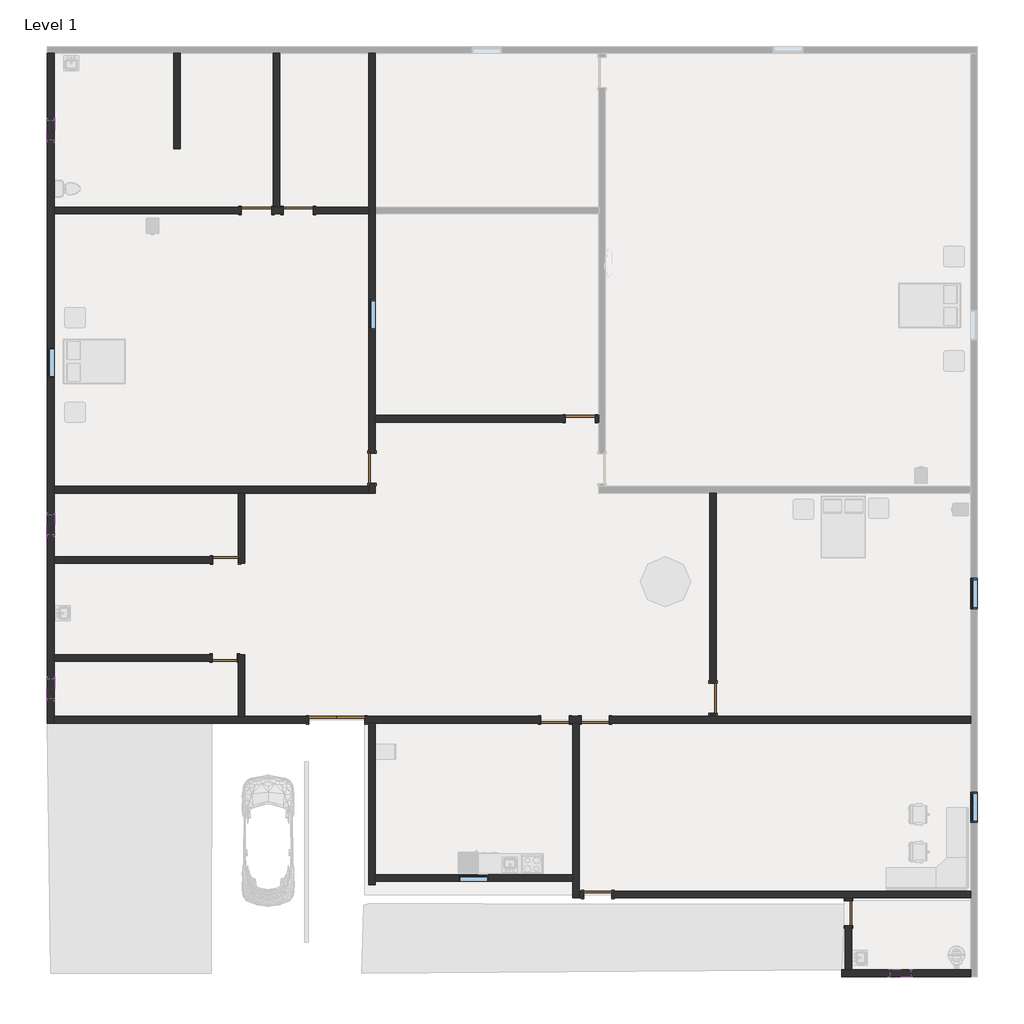
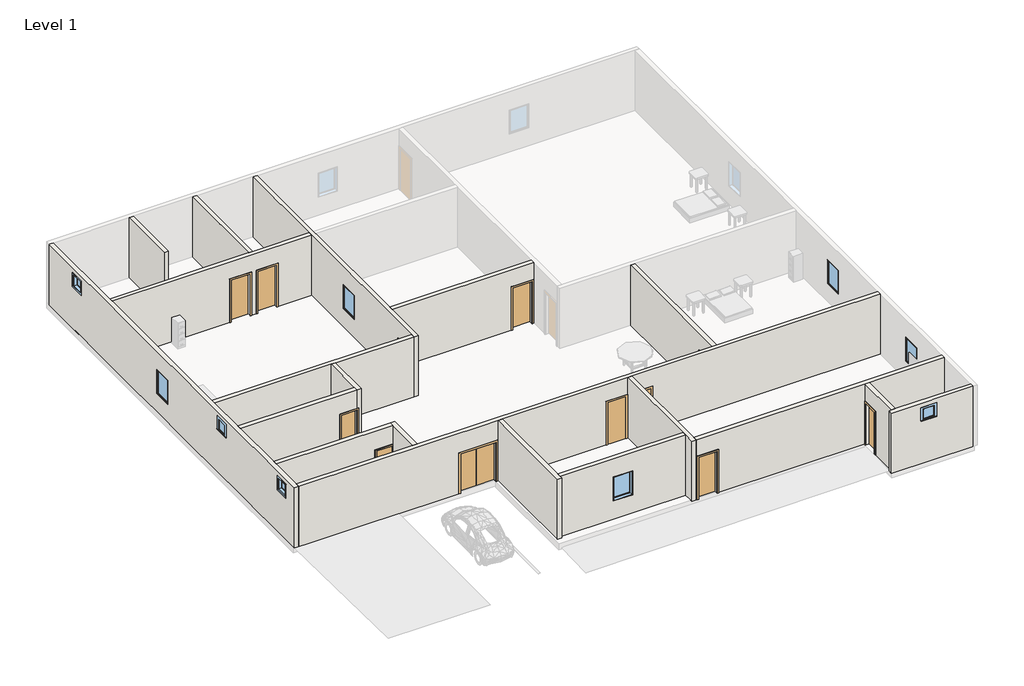
# One storey, part 1 of 2: 19 walls, 12 doors, 9 windows.
"""IFC4 building model written with IfcOpenShell, lengths in millimetres."""

from ifc_helpers import new_model, si_unit, frame, origin, origin_with_axes, place, context, project, spatial, polyline, outline, extrude, faceted_brep, transform, mapped, element, save
from components import m_door_double_flush_panel_1700_x_2000mm_97be971e, door_fadea3f2, door_53b1b562, door_4314e8ec, door_74220ae7, door_f75d31f8, door_54dd4da4, door_719f80de, window_e2841890, window_e41d21a6

model = new_model("IFC4")

# Units and contexts
model_context = context("Model", 3, world=origin())
ifc_project = project(units=[si_unit("LENGTHUNIT", "METRE", prefix="MILLI")], contexts=[model_context])

# Site, building, storey
site = spatial("IfcSite", under=ifc_project)
building = spatial("IfcBuilding", under=site)
storey = spatial("IfcBuildingStorey", under=building, Name="Level 1", Elevation=0.0)

# Doors
placement = place(None, origin())
m_door_double_flush_panel_1700_x_2000mm_shape = m_door_double_flush_panel_1700_x_2000mm_97be971e(model_context)
element("IfcDoor", 1, ObjectType="M_Door-Double-Flush_Panel : 1700 x 2000mm", at=placement, inside=storey, context=model_context, shape_type="MappedRepresentation", body=[
    mapped(m_door_double_flush_panel_1700_x_2000mm_shape, transform((-7405.8725091, -4969.7754008, 0.0), x_axis=(1.0, 0.0, 0.0), y_axis=(0.0, 1.0, 0.0), z_axis=(0.0, 0.0, 1.0))),
])
door_shape = door_fadea3f2(model_context)
element("IfcDoor", 2, ObjectType="Single-Flush : 30\" x 80\"", at=placement, inside=storey, context=model_context, shape_type="MappedRepresentation", body=[
    mapped(door_shape, transform((-10784.0725091, -118.3754008, 0.0), x_axis=(1.0, 0.0, 0.0), y_axis=(0.0, 1.0, 0.0), z_axis=(0.0, 0.0, 1.0))),
])
door_2_shape = door_53b1b562(model_context)
element("IfcDoor", 3, ObjectType="Single-Flush : 30\" x 80\"", at=placement, inside=storey, context=model_context, shape_type="MappedRepresentation", body=[
    mapped(door_2_shape, transform((-10809.4725091, -3090.1754008, 0.0), x_axis=(1.0, 0.0, 0.0), y_axis=(0.0, 1.0, 0.0), z_axis=(0.0, 0.0, 1.0))),
])
door_3_shape = door_4314e8ec(model_context)
element("IfcDoor", 4, ObjectType="Single-Flush : 30\" x 84\"", at=placement, inside=storey, context=model_context, shape_type="MappedRepresentation", body=[
    mapped(door_3_shape, transform((8138.9274909, -10837.1754008, 0.0), x_axis=(0.0, 1.0, 0.0), y_axis=(-1.0, 0.0, 0.0), z_axis=(0.0, 0.0, 1.0))),
])
door_4_shape = door_74220ae7(model_context)
element("IfcDoor", 5, ObjectType="Single-Flush : 34\" x 84\"", at=placement, inside=storey, context=model_context, shape_type="MappedRepresentation", body=[
    mapped(door_4_shape, transform((-776.4725091, -4969.7754008, 0.0), x_axis=(1.0, 0.0, 0.0), y_axis=(0.0, 1.0, 0.0), z_axis=(0.0, 0.0, 1.0))),
])
element("IfcDoor", 6, ObjectType="Single-Flush : 34\" x 84\"", at=placement, inside=storey, context=model_context, shape_type="MappedRepresentation", body=[
    mapped(door_4_shape, transform((518.9274909, -10278.3754008, 0.0), x_axis=(-1.0, 0.0, 0.0), y_axis=(0.0, -1.0, 0.0), z_axis=(0.0, 0.0, 1.0))),
])
door_5_shape = door_f75d31f8(model_context)
element("IfcDoor", 7, ObjectType="Single-Flush : 34\" x 84\"", at=placement, inside=storey, context=model_context, shape_type="MappedRepresentation", body=[
    mapped(door_5_shape, transform((442.7274909, -4969.7754008, 0.0), x_axis=(-1.0, 0.0, 0.0), y_axis=(0.0, -1.0, 0.0), z_axis=(0.0, 0.0, 1.0))),
])
door_6_shape = door_54dd4da4(model_context)
element("IfcDoor", 8, ObjectType="Single-Flush : 36\" x 84\"", at=placement, inside=storey, context=model_context, shape_type="MappedRepresentation", body=[
    mapped(door_6_shape, transform((-9844.2725091, 10498.8245992, 0.0), x_axis=(1.0, 0.0, 0.0), y_axis=(0.0, 1.0, 0.0), z_axis=(0.0, 0.0, 1.0))),
])
element("IfcDoor", 9, ObjectType="Single-Flush : 36\" x 84\"", at=placement, inside=storey, context=model_context, shape_type="MappedRepresentation", body=[
    mapped(door_6_shape, transform((-14.4725091, 4174.2245992, 0.0), x_axis=(1.0, 0.0, 0.0), y_axis=(0.0, 1.0, 0.0), z_axis=(0.0, 0.0, 1.0))),
])
element("IfcDoor", 10, ObjectType="Single-Flush : 36\" x 84\"", at=placement, inside=storey, context=model_context, shape_type="MappedRepresentation", body=[
    mapped(door_6_shape, transform((4024.1274909, -4309.3754008, 0.0), x_axis=(0.0, -1.0, 0.0), y_axis=(1.0, 0.0, 0.0), z_axis=(0.0, 0.0, 1.0))),
])
door_7_shape = door_719f80de(model_context)
element("IfcDoor", 11, ObjectType="Single-Flush : 36\" x 84\"", at=placement, inside=storey, context=model_context, shape_type="MappedRepresentation", body=[
    mapped(door_7_shape, transform((-8574.2725091, 10498.8245992, 0.0), x_axis=(-1.0, 0.0, 0.0), y_axis=(0.0, -1.0, 0.0), z_axis=(0.0, 0.0, 1.0))),
])
element("IfcDoor", 12, ObjectType="Single-Flush : 36\" x 84\"", at=placement, inside=storey, context=model_context, shape_type="MappedRepresentation", body=[
    mapped(door_7_shape, transform((-6339.0725091, 2675.6245992, 0.0), x_axis=(0.0, -1.0, 0.0), y_axis=(1.0, 0.0, 0.0), z_axis=(0.0, 0.0, 1.0))),
])

# Walls
element("IfcWall", 13, ObjectType="Generic - 8\"", at=placement, inside=storey, context=model_context, shape_type="Brep", body=[
    faceted_brep([(11847.3274909, -12564.3754008, 0.0), (8240.5274909, -12564.3754008, 0.0), (8037.3274909, -12564.3754008, 0.0), (7935.7274909, -12564.3754008, 0.0), (7935.7274909, -12564.3754008, 3048.0), (8037.3274909, -12564.3754008, 3048.0), (8240.5274909, -12564.3754008, 3048.0), (11847.3274909, -12564.3754008, 3048.0), (9408.9274909, -12564.3754008, 2768.6), (9408.9274909, -12564.3754008, 2159.0), (10018.5274909, -12564.3754008, 2159.0), (10018.5274909, -12564.3754008, 2768.6), (11847.3274909, -12767.5754008, 0.0), (11847.3274909, -12767.5754008, 3048.0), (7935.7274909, -12767.5754008, 3048.0), (7935.7274909, -12767.5754008, 0.0), (9408.9274909, -12767.5754008, 2768.6), (10018.5274909, -12767.5754008, 2768.6), (10018.5274909, -12767.5754008, 2159.0), (9408.9274909, -12767.5754008, 2159.0)], [[[0, 1, 2, 3, 4, 5, 6, 7], [8, 9, 10, 11]], [[12, 13, 14, 15], [16, 17, 18, 19]], [[3, 2, 1, 0, 12, 15]], [[4, 3, 15, 14]], [[7, 6, 5, 4, 14, 13]], [[0, 7, 13, 12]], [[9, 8, 16, 19]], [[10, 9, 19, 18]], [[11, 10, 18, 17]], [[8, 11, 17, 16]]]),
])
element("IfcWall", 14, ObjectType="Generic - 8\"", at=placement, inside=storey, context=model_context, shape_type="Brep", body=[
    faceted_brep([(-6440.6725091, 2218.4245992, 2133.6), (-6440.6725091, 2218.4245992, 0.0), (-6440.6725091, 2116.8245992, 0.0), (-6440.6725091, 1913.6245992, 0.0), (-6440.6725091, 1913.6245992, 3048.0), (-6440.6725091, 2116.8245992, 3048.0), (-6440.6725091, 10397.2245992, 3048.0), (-6440.6725091, 10600.4245992, 3048.0), (-6440.6725091, 15274.0245992, 3048.0), (-6440.6725091, 15274.0245992, 0.0), (-6440.6725091, 10600.4245992, 0.0), (-6440.6725091, 10397.2245992, 0.0), (-6440.6725091, 3132.8245992, 0.0), (-6440.6725091, 3132.8245992, 2133.6), (-6440.6725091, 7793.7245992, 2133.6), (-6440.6725091, 6879.3245992, 2133.6), (-6440.6725091, 6879.3245992, 914.4), (-6440.6725091, 7793.7245992, 914.4), (-6237.4725091, 1913.6245992, 0.0), (-6237.4725091, 2218.4245992, 0.0), (-6237.4725091, 2218.4245992, 2133.6), (-6237.4725091, 3132.8245992, 2133.6), (-6237.4725091, 3132.8245992, 0.0), (-6237.4725091, 4072.6245992, 0.0), (-6237.4725091, 4275.8245992, 0.0), (-6237.4725091, 10397.2245992, 0.0), (-6237.4725091, 10600.4245992, 0.0), (-6237.4725091, 15274.0245992, 0.0), (-6237.4725091, 15274.0245992, 3048.0), (-6237.4725091, 10600.4245992, 3048.0), (-6237.4725091, 10397.2245992, 3048.0), (-6237.4725091, 4275.8245992, 3048.0), (-6237.4725091, 4072.6245992, 3048.0), (-6237.4725091, 1913.6245992, 3048.0), (-6237.4725091, 7793.7245992, 2133.6), (-6237.4725091, 7793.7245992, 914.4), (-6237.4725091, 6879.3245992, 914.4), (-6237.4725091, 6879.3245992, 2133.6)], [[[0, 1, 2, 3, 4, 5, 6, 7, 8, 9, 10, 11, 12, 13], [14, 15, 16, 17]], [[18, 19, 20, 21, 22, 23, 24, 25, 26, 27, 28, 29, 30, 31, 32, 33], [34, 35, 36, 37]], [[3, 2, 1, 19, 18]], [[12, 11, 10, 9, 27, 26, 25, 24, 23, 22]], [[8, 7, 6, 5, 4, 33, 32, 31, 30, 29, 28]], [[9, 8, 28, 27]], [[4, 3, 18, 33]], [[20, 19, 1, 0]], [[21, 20, 0, 13]], [[22, 21, 13, 12]], [[35, 34, 14, 17]], [[36, 35, 17, 16]], [[37, 36, 16, 15]], [[34, 37, 15, 14]]]),
])
element("IfcWall", 15, ObjectType="Generic - 8\"", at=placement, inside=storey, context=model_context, shape_type="Brep", body=[
    faceted_brep([(-9031.4725091, 10600.4245992, 2133.6), (-9031.4725091, 10600.4245992, 0.0), (-9133.0725091, 10600.4245992, 0.0), (-9336.2725091, 10600.4245992, 0.0), (-9387.0725091, 10600.4245992, 0.0), (-9387.0725091, 10600.4245992, 2133.6), (-10301.4725091, 10600.4245992, 2133.6), (-10301.4725091, 10600.4245992, 0.0), (-15991.0725091, 10600.4245992, 0.0), (-15991.0725091, 10600.4245992, 3048.0), (-9336.2725091, 10600.4245992, 3048.0), (-9133.0725091, 10600.4245992, 3048.0), (-6440.6725091, 10600.4245992, 3048.0), (-6440.6725091, 10600.4245992, 0.0), (-8117.0725091, 10600.4245992, 0.0), (-8117.0725091, 10600.4245992, 2133.6), (-9387.0725091, 10397.2245992, 0.0), (-9031.4725091, 10397.2245992, 0.0), (-9031.4725091, 10397.2245992, 2133.6), (-8117.0725091, 10397.2245992, 2133.6), (-8117.0725091, 10397.2245992, 0.0), (-6440.6725091, 10397.2245992, 0.0), (-6440.6725091, 10397.2245992, 3048.0), (-15991.0725091, 10397.2245992, 3048.0), (-15991.0725091, 10397.2245992, 0.0), (-10301.4725091, 10397.2245992, 0.0), (-10301.4725091, 10397.2245992, 2133.6), (-9387.0725091, 10397.2245992, 2133.6)], [[[0, 1, 2, 3, 4, 5, 6, 7, 8, 9, 10, 11, 12, 13, 14, 15]], [[16, 17, 18, 19, 20, 21, 22, 23, 24, 25, 26, 27]], [[25, 24, 8, 7]], [[14, 13, 21, 20]], [[4, 3, 2, 1, 17, 16]], [[12, 11, 10, 9, 23, 22]], [[13, 12, 22, 21]], [[9, 8, 24, 23]], [[5, 4, 16, 27]], [[6, 5, 27, 26]], [[7, 6, 26, 25]], [[18, 17, 1, 0]], [[19, 18, 0, 15]], [[20, 19, 15, 14]]]),
])
element("IfcWall", 16, ObjectType="Generic - 8\"", at=placement, inside=storey, context=model_context, shape_type="Brep", body=[
    faceted_brep([(-6440.6725091, 2116.8245992, 0.0), (-15991.0725091, 2116.8245992, 0.0), (-15991.0725091, 2116.8245992, 3048.0), (-6440.6725091, 2116.8245992, 3048.0), (-6440.6725091, 1913.6245992, 0.0), (-6440.6725091, 1913.6245992, 3048.0), (-10199.8725091, 1913.6245992, 3048.0), (-10403.0725091, 1913.6245992, 3048.0), (-15991.0725091, 1913.6245992, 3048.0), (-15991.0725091, 1913.6245992, 0.0), (-10403.0725091, 1913.6245992, 0.0), (-10199.8725091, 1913.6245992, 0.0)], [[[0, 1, 2, 3]], [[4, 5, 6, 7, 8, 9, 10, 11]], [[1, 0, 4, 11, 10, 9]], [[3, 2, 8, 7, 6, 5]], [[0, 3, 5, 4]], [[2, 1, 9, 8]]]),
])
element("IfcWall", 17, ObjectType="Generic - 8\"", at=placement, inside=storey, context=model_context, shape_type="Brep", body=[
    faceted_brep([(-10403.0725091, 1913.6245992, 0.0), (-10403.0725091, -219.9754008, 0.0), (-10403.0725091, -219.9754008, 2032.0), (-10403.0725091, -219.9754008, 3048.0), (-10403.0725091, -16.7754008, 3048.0), (-10403.0725091, 1913.6245992, 3048.0), (-10199.8725091, 1913.6245992, 0.0), (-10199.8725091, 1913.6245992, 3048.0), (-10199.8725091, -219.9754008, 3048.0), (-10199.8725091, -219.9754008, 0.0)], [[[0, 1, 2, 3, 4, 5]], [[6, 7, 8, 9]], [[1, 0, 6, 9]], [[5, 4, 3, 8, 7]], [[0, 5, 7, 6]], [[3, 2, 1, 9, 8]]]),
])
element("IfcWall", 18, ObjectType="Generic - 8\"", at=placement, inside=storey, context=model_context, shape_type="Brep", body=[
    faceted_brep([(10.9274909, -4868.1754008, 2133.6), (10.9274909, -4868.1754008, 0.0), (-344.6725091, -4868.1754008, 0.0), (-344.6725091, -4868.1754008, 2133.6), (-1208.2725091, -4868.1754008, 2133.6), (-1208.2725091, -4868.1754008, 0.0), (-6555.8725091, -4868.1754008, 0.0), (-6555.8725091, -4868.1754008, 2000.0), (-8255.8725091, -4868.1754008, 2000.0), (-8255.8725091, -4868.1754008, 0.0), (-10199.8725091, -4868.1754008, 0.0), (-10403.0725091, -4868.1754008, 0.0), (-15991.0725091, -4868.1754008, 0.0), (-15991.0725091, -4868.1754008, 3048.0), (-10403.0725091, -4868.1754008, 3048.0), (-10199.8725091, -4868.1754008, 3048.0), (3922.5274909, -4868.1754008, 3048.0), (4125.7274909, -4868.1754008, 3048.0), (11847.3274909, -4868.1754008, 3048.0), (11847.3274909, -4868.1754008, 0.0), (4125.7274909, -4868.1754008, 0.0), (3922.5274909, -4868.1754008, 0.0), (874.5274909, -4868.1754008, 0.0), (874.5274909, -4868.1754008, 2133.6), (-344.6725091, -5071.3754008, 0.0), (-243.0725091, -5071.3754008, 0.0), (-39.8725091, -5071.3754008, 0.0), (10.9274909, -5071.3754008, 0.0), (10.9274909, -5071.3754008, 2133.6), (874.5274909, -5071.3754008, 2133.6), (874.5274909, -5071.3754008, 0.0), (11847.3274909, -5071.3754008, 0.0), (11847.3274909, -5071.3754008, 3048.0), (-39.8725091, -5071.3754008, 3048.0), (-243.0725091, -5071.3754008, 3048.0), (-6237.4725091, -5071.3754008, 3048.0), (-6440.6725091, -5071.3754008, 3048.0), (-15991.0725091, -5071.3754008, 3048.0), (-15991.0725091, -5071.3754008, 0.0), (-8255.8725091, -5071.3754008, 0.0), (-8255.8725091, -5071.3754008, 2000.0), (-6555.8725091, -5071.3754008, 2000.0), (-6555.8725091, -5071.3754008, 0.0), (-6440.6725091, -5071.3754008, 0.0), (-6237.4725091, -5071.3754008, 0.0), (-1208.2725091, -5071.3754008, 0.0), (-1208.2725091, -5071.3754008, 2133.6), (-344.6725091, -5071.3754008, 2133.6)], [[[0, 1, 2, 3, 4, 5, 6, 7, 8, 9, 10, 11, 12, 13, 14, 15, 16, 17, 18, 19, 20, 21, 22, 23]], [[24, 25, 26, 27, 28, 29, 30, 31, 32, 33, 34, 35, 36, 37, 38, 39, 40, 41, 42, 43, 44, 45, 46, 47]], [[38, 12, 11, 10, 9, 39]], [[45, 44, 43, 42, 6, 5]], [[2, 1, 27, 26, 25, 24]], [[22, 21, 20, 19, 31, 30]], [[18, 17, 16, 15, 14, 13, 37, 36, 35, 34, 33, 32]], [[19, 18, 32, 31]], [[41, 7, 6, 42]], [[7, 41, 40, 8]], [[8, 40, 39, 9]], [[13, 12, 38, 37]], [[3, 2, 24, 47]], [[4, 3, 47, 46]], [[5, 4, 46, 45]], [[28, 27, 1, 0]], [[29, 28, 0, 23]], [[30, 29, 23, 22]]]),
])
element("IfcWall", 19, ObjectType="Generic - 8\"", at=placement, inside=storey, context=model_context, shape_type="Brep", body=[
    faceted_brep([(-6440.6725091, -5071.3754008, 0.0), (-6440.6725091, -9973.5754008, 0.0), (-6440.6725091, -9973.5754008, 3048.0), (-6440.6725091, -5071.3754008, 3048.0), (-6237.4725091, -5071.3754008, 0.0), (-6237.4725091, -5071.3754008, 3048.0), (-6237.4725091, -9668.7754008, 3048.0), (-6237.4725091, -9871.9754008, 3048.0), (-6237.4725091, -9973.5754008, 3048.0), (-6237.4725091, -9973.5754008, 0.0), (-6237.4725091, -9871.9754008, 0.0), (-6237.4725091, -9668.7754008, 0.0)], [[[0, 1, 2, 3]], [[4, 5, 6, 7, 8, 9, 10, 11]], [[1, 0, 4, 11, 10, 9]], [[2, 1, 9, 8]], [[3, 2, 8, 7, 6, 5]], [[0, 3, 5, 4]]]),
])
element("IfcWall", 20, ObjectType="Generic - 8\"", at=placement, inside=storey, context=model_context, shape_type="Brep", body=[
    faceted_brep([(-243.0725091, -5071.3754008, 0.0), (-243.0725091, -9668.7754008, 0.0), (-243.0725091, -9871.9754008, 0.0), (-243.0725091, -10379.9754008, 0.0), (-243.0725091, -10379.9754008, 3048.0), (-243.0725091, -9871.9754008, 3048.0), (-243.0725091, -9668.7754008, 3048.0), (-243.0725091, -5071.3754008, 3048.0), (-39.8725091, -5071.3754008, 0.0), (-39.8725091, -5071.3754008, 3048.0), (-39.8725091, -10176.7754008, 3048.0), (-39.8725091, -10379.9754008, 3048.0), (-39.8725091, -10379.9754008, 0.0), (-39.8725091, -10176.7754008, 0.0)], [[[0, 1, 2, 3, 4, 5, 6, 7]], [[8, 9, 10, 11, 12, 13]], [[3, 2, 1, 0, 8, 13, 12]], [[7, 6, 5, 4, 11, 10, 9]], [[0, 7, 9, 8]], [[4, 3, 12, 11]]]),
])
element("IfcWall", 21, ObjectType="Generic - 8\"", at=placement, inside=storey, context=model_context, shape_type="SweptSolid", body=[
    extrude(outline(polyline([(0.0, -6237.4725091), (0.0, -243.0725091), (3048.0, -243.0725091), (3048.0, -6237.4725091), (0.0, -6237.4725091)]), holes=[polyline([(2133.6, -2783.0725091), (914.4, -2783.0725091), (914.4, -3697.4725091), (2133.6, -3697.4725091), (2133.6, -2783.0725091)])]), frame((0.0, -9871.9754008, 0.0), z_axis=(0.0, 1.0, 0.0), x_axis=(0.0, 0.0, 1.0)), (0.0, 0.0, 1.0), 203.2),
])
element("IfcWall", 22, ObjectType="Generic - 8\"", at=placement, inside=storey, context=model_context, shape_type="Brep", body=[
    faceted_brep([(-39.8725091, -10379.9754008, 0.0), (87.1274909, -10379.9754008, 0.0), (87.1274909, -10379.9754008, 2133.6), (950.7274909, -10379.9754008, 2133.6), (950.7274909, -10379.9754008, 0.0), (8037.3274909, -10379.9754008, 0.0), (8240.5274909, -10379.9754008, 0.0), (11847.3274909, -10379.9754008, 0.0), (11847.3274909, -10379.9754008, 3048.0), (8240.5274909, -10379.9754008, 3048.0), (8037.3274909, -10379.9754008, 3048.0), (-39.8725091, -10379.9754008, 3048.0), (87.1274909, -10176.7754008, 2133.6), (87.1274909, -10176.7754008, 0.0), (-39.8725091, -10176.7754008, 0.0), (-39.8725091, -10176.7754008, 3048.0), (11847.3274909, -10176.7754008, 3048.0), (11847.3274909, -10176.7754008, 0.0), (950.7274909, -10176.7754008, 0.0), (950.7274909, -10176.7754008, 2133.6)], [[[0, 1, 2, 3, 4, 5, 6, 7, 8, 9, 10, 11]], [[12, 13, 14, 15, 16, 17, 18, 19]], [[18, 17, 7, 6, 5, 4]], [[14, 13, 1, 0]], [[11, 10, 9, 8, 16, 15]], [[0, 11, 15, 14]], [[8, 7, 17, 16]], [[2, 1, 13, 12]], [[3, 2, 12, 19]], [[4, 3, 19, 18]]]),
])
element("IfcWall", 23, ObjectType="Generic - 8\"", at=placement, inside=storey, context=model_context, shape_type="SweptSolid", body=[
    extrude(outline(polyline([(-10379.9754008, 0.0), (-10456.1754008, 0.0), (-10456.1754008, 2133.6), (-11218.1754008, 2133.6), (-11218.1754008, 0.0), (-12564.3754008, 0.0), (-12564.3754008, 3048.0), (-10379.9754008, 3048.0), (-10379.9754008, 0.0)])), frame((8037.3274909, 0.0, 0.0), z_axis=(1.0, 0.0, 0.0), x_axis=(0.0, 1.0, 0.0)), (0.0, 0.0, 1.0), 203.2),
])
element("IfcWall", 24, ObjectType="Generic - 8\"", at=placement, inside=storey, context=model_context, shape_type="SweptSolid", body=[
    extrude(outline(polyline([(2133.6, 442.7274909), (0.0, 442.7274909), (0.0, 544.3274909), (3048.0, 544.3274909), (3048.0, -6237.4725091), (0.0, -6237.4725091), (0.0, -471.6725091), (2133.6, -471.6725091), (2133.6, 442.7274909)])), frame((0.0, 4072.6245992, 0.0), z_axis=(0.0, 1.0, 0.0), x_axis=(0.0, 0.0, 1.0)), (0.0, 0.0, 1.0), 203.2),
])
element("IfcWall", 25, ObjectType="Generic - 8\"", at=placement, inside=storey, context=model_context, shape_type="SweptSolid", body=[
    extrude(outline(polyline([(-12358.8725091, 12378.4245992), (-12358.8725091, 15274.0245992), (-12155.6725091, 15274.0245992), (-12155.6725091, 12378.4245992), (-12358.8725091, 12378.4245992)])), origin_with_axes(), (0.0, 0.0, 1.0), 3048.0),
])
element("IfcWall", 26, ObjectType="Generic - 8\"", at=placement, inside=storey, context=model_context, shape_type="SweptSolid", body=[
    extrude(outline(polyline([(-9336.2725091, 10600.4245992), (-9336.2725091, 15274.0245992), (-9133.0725091, 15274.0245992), (-9133.0725091, 10600.4245992), (-9336.2725091, 10600.4245992)])), origin_with_axes(), (0.0, 0.0, 1.0), 3048.0),
])
element("IfcWall", 27, ObjectType="Generic - 8\"", at=placement, inside=storey, context=model_context, shape_type="SweptSolid", body=[
    extrude(outline(polyline([(-4766.5754008, 2133.6), (-4766.5754008, 0.0), (-4868.1754008, 0.0), (-4868.1754008, 3048.0), (1913.6245992, 3048.0), (1913.6245992, 0.0), (-3852.1754008, 0.0), (-3852.1754008, 2133.6), (-4766.5754008, 2133.6)])), frame((3922.5274909, 0.0, 0.0), z_axis=(1.0, 0.0, 0.0), x_axis=(0.0, 1.0, 0.0)), (0.0, 0.0, 1.0), 203.2),
])
element("IfcWall", 28, ObjectType="Generic - 8\"", at=placement, inside=storey, context=model_context, shape_type="Brep", body=[
    faceted_brep([(-10403.0725091, -2988.5754008, 0.0), (-10403.0725091, -3191.7754008, 0.0), (-10403.0725091, -4868.1754008, 0.0), (-10403.0725091, -4868.1754008, 3048.0), (-10403.0725091, -3191.7754008, 3048.0), (-10403.0725091, -2988.5754008, 3048.0), (-10199.8725091, -2988.5754008, 0.0), (-10199.8725091, -2988.5754008, 3048.0), (-10199.8725091, -4868.1754008, 3048.0), (-10199.8725091, -4868.1754008, 0.0)], [[[0, 1, 2, 3, 4, 5]], [[6, 7, 8, 9]], [[2, 1, 0, 6, 9]], [[5, 4, 3, 8, 7]], [[3, 2, 9, 8]], [[0, 5, 7, 6]]]),
])
element("IfcWall", 29, ObjectType="Generic - 8\"", at=placement, inside=storey, context=model_context, shape_type="SweptSolid", body=[
    extrude(outline(polyline([(3048.0, -10403.0725091), (3048.0, -15991.0725091), (0.0, -15991.0725091), (0.0, -11165.0725091), (2032.0, -11165.0725091), (2032.0, -10403.0725091), (3048.0, -10403.0725091)])), frame((0.0, -219.9754008, 0.0), z_axis=(0.0, 1.0, 0.0), x_axis=(0.0, 0.0, 1.0)), (0.0, 0.0, 1.0), 203.2),
])
element("IfcWall", 30, ObjectType="Generic - 8\"", at=placement, inside=storey, context=model_context, shape_type="SweptSolid", body=[
    extrude(outline(polyline([(2032.0, -10428.4725091), (0.0, -10428.4725091), (0.0, -10403.0725091), (3048.0, -10403.0725091), (3048.0, -15991.0725091), (0.0, -15991.0725091), (0.0, -11190.4725091), (2032.0, -11190.4725091), (2032.0, -10428.4725091)])), frame((0.0, -3191.7754008, 0.0), z_axis=(0.0, 1.0, 0.0), x_axis=(0.0, 0.0, 1.0)), (0.0, 0.0, 1.0), 203.2),
])
element("IfcWall", 31, ObjectType="Generic - 8\"", at=placement, inside=storey, context=model_context, shape_type="Brep", body=[
    faceted_brep([(-15991.0725091, -5071.3754008, 0.0), (-15991.0725091, -4868.1754008, 0.0), (-15991.0725091, -3191.7754008, 0.0), (-15991.0725091, -2988.5754008, 0.0), (-15991.0725091, -219.9754008, 0.0), (-15991.0725091, -16.7754008, 0.0), (-15991.0725091, 1913.6245992, 0.0), (-15991.0725091, 2116.8245992, 0.0), (-15991.0725091, 10397.2245992, 0.0), (-15991.0725091, 10600.4245992, 0.0), (-15991.0725091, 15274.0245992, 0.0), (-15991.0725091, 15274.0245992, 3048.0), (-15991.0725091, 10600.4245992, 3048.0), (-15991.0725091, 10397.2245992, 3048.0), (-15991.0725091, 2116.8245992, 3048.0), (-15991.0725091, 1913.6245992, 3048.0), (-15991.0725091, -16.7754008, 3048.0), (-15991.0725091, -219.9754008, 3048.0), (-15991.0725091, -2988.5754008, 3048.0), (-15991.0725091, -3191.7754008, 3048.0), (-15991.0725091, -4868.1754008, 3048.0), (-15991.0725091, -5071.3754008, 3048.0), (-15991.0725091, 6333.2245992, 2133.6), (-15991.0725091, 6333.2245992, 914.4), (-15991.0725091, 5418.8245992, 914.4), (-15991.0725091, 5418.8245992, 2133.6), (-15991.0725091, -4334.7754008, 2768.6), (-15991.0725091, -3725.1754008, 2768.6), (-15991.0725091, -3725.1754008, 2159.0), (-15991.0725091, -4334.7754008, 2159.0), (-15991.0725091, 1253.2245992, 2768.6), (-15991.0725091, 1253.2245992, 2159.0), (-15991.0725091, 643.6245992, 2159.0), (-15991.0725091, 643.6245992, 2768.6), (-15991.0725091, 12632.4245992, 2768.6), (-15991.0725091, 13242.0245992, 2768.6), (-15991.0725091, 13242.0245992, 2159.0), (-15991.0725091, 12632.4245992, 2159.0), (-16194.2725091, -5071.3754008, 0.0), (-16194.2725091, -5071.3754008, 3048.0), (-16194.2725091, 15274.0245992, 3048.0), (-16194.2725091, 15274.0245992, 0.0), (-16194.2725091, 6333.2245992, 2133.6), (-16194.2725091, 5418.8245992, 2133.6), (-16194.2725091, 5418.8245992, 914.4), (-16194.2725091, 6333.2245992, 914.4), (-16194.2725091, -4334.7754008, 2768.6), (-16194.2725091, -4334.7754008, 2159.0), (-16194.2725091, -3725.1754008, 2159.0), (-16194.2725091, -3725.1754008, 2768.6), (-16194.2725091, 1253.2245992, 2768.6), (-16194.2725091, 643.6245992, 2768.6), (-16194.2725091, 643.6245992, 2159.0), (-16194.2725091, 1253.2245992, 2159.0), (-16194.2725091, 12632.4245992, 2768.6), (-16194.2725091, 12632.4245992, 2159.0), (-16194.2725091, 13242.0245992, 2159.0), (-16194.2725091, 13242.0245992, 2768.6)], [[[0, 1, 2, 3, 4, 5, 6, 7, 8, 9, 10, 11, 12, 13, 14, 15, 16, 17, 18, 19, 20, 21], [22, 23, 24, 25], [26, 27, 28, 29], [30, 31, 32, 33], [34, 35, 36, 37]], [[38, 39, 40, 41], [42, 43, 44, 45], [46, 47, 48, 49], [50, 51, 52, 53], [54, 55, 56, 57]], [[10, 9, 8, 7, 6, 5, 4, 3, 2, 1, 0, 38, 41]], [[21, 20, 19, 18, 17, 16, 15, 14, 13, 12, 11, 40, 39]], [[11, 10, 41, 40]], [[0, 21, 39, 38]], [[23, 22, 42, 45]], [[24, 23, 45, 44]], [[25, 24, 44, 43]], [[22, 25, 43, 42]], [[47, 46, 26, 29]], [[48, 47, 29, 28]], [[49, 48, 28, 27]], [[46, 49, 27, 26]], [[31, 30, 50, 53]], [[32, 31, 53, 52]], [[33, 32, 52, 51]], [[30, 33, 51, 50]], [[55, 54, 34, 37]], [[56, 55, 37, 36]], [[57, 56, 36, 35]], [[54, 57, 35, 34]]]),
])

# Windows
window_shape = window_e2841890(model_context)
element("IfcWindow", 32, ObjectType="Fixed : 36\" x 48\"", at=placement, inside=storey, context=model_context, shape_type="MappedRepresentation", body=[
    mapped(window_shape, transform((-16092.6725091, 5914.1245992, 0.0), x_axis=(0.0, 1.0, 0.0), y_axis=(-1.0, 0.0, 0.0), z_axis=(0.0, 0.0, 1.0))),
])
element("IfcWindow", 33, ObjectType="Fixed : 36\" x 48\"", at=placement, inside=storey, context=model_context, shape_type="MappedRepresentation", body=[
    mapped(window_shape, transform((-3202.1725091, -9770.3754008, 0.0), x_axis=(1.0, 0.0, 0.0), y_axis=(0.0, 1.0, 0.0), z_axis=(0.0, 0.0, 1.0))),
])
element("IfcWindow", 34, ObjectType="Fixed : 36\" x 48\"", at=placement, inside=storey, context=model_context, shape_type="MappedRepresentation", body=[
    mapped(window_shape, transform((11948.9274909, -7585.9754008, 0.0), x_axis=(0.0, 1.0, 0.0), y_axis=(-1.0, 0.0, 0.0), z_axis=(0.0, 0.0, 1.0))),
])
element("IfcWindow", 35, ObjectType="Fixed : 36\" x 48\"", at=placement, inside=storey, context=model_context, shape_type="MappedRepresentation", body=[
    mapped(window_shape, transform((11948.9274909, -1096.2754008, 0.0), x_axis=(0.0, 1.0, 0.0), y_axis=(-1.0, 0.0, 0.0), z_axis=(0.0, 0.0, 1.0))),
])
element("IfcWindow", 36, ObjectType="Fixed : 36\" x 48\"", at=placement, inside=storey, context=model_context, shape_type="MappedRepresentation", body=[
    mapped(window_shape, transform((-6339.0725091, 7374.6245992, 0.0), x_axis=(0.0, 1.0, 0.0), y_axis=(-1.0, 0.0, 0.0), z_axis=(0.0, 0.0, 1.0))),
])
window_2_shape = window_e41d21a6(model_context)
element("IfcWindow", 37, ObjectType="Transom with Trim : 24\" x 24\"", at=placement, inside=storey, context=model_context, shape_type="MappedRepresentation", body=[
    mapped(window_2_shape, transform((-16092.6725091, -4068.0754008, 0.0), x_axis=(0.0, -1.0, 0.0), y_axis=(1.0, 0.0, 0.0), z_axis=(0.0, 0.0, 1.0))),
])
element("IfcWindow", 38, ObjectType="Transom with Trim : 24\" x 24\"", at=placement, inside=storey, context=model_context, shape_type="MappedRepresentation", body=[
    mapped(window_2_shape, transform((-16092.6725091, 986.5245992, 0.0), x_axis=(0.0, 1.0, 0.0), y_axis=(-1.0, 0.0, 0.0), z_axis=(0.0, 0.0, 1.0))),
])
element("IfcWindow", 39, ObjectType="Transom with Trim : 24\" x 24\"", at=placement, inside=storey, context=model_context, shape_type="MappedRepresentation", body=[
    mapped(window_2_shape, transform((-16092.6725091, 12899.1245992, 0.0), x_axis=(0.0, -1.0, 0.0), y_axis=(1.0, 0.0, 0.0), z_axis=(0.0, 0.0, 1.0))),
])
element("IfcWindow", 40, ObjectType="Transom with Trim : 24\" x 24\"", at=placement, inside=storey, context=model_context, shape_type="MappedRepresentation", body=[
    mapped(window_2_shape, transform((9675.6274909, -12665.9754008, 0.0), x_axis=(-1.0, 0.0, 0.0), y_axis=(0.0, -1.0, 0.0), z_axis=(0.0, 0.0, 1.0))),
])

save(model, "model.ifc")

# Revit data of these elements
# Type "M_Door-Double-Flush_Panel : 1700 x 2000mm"
#   Type Mark = "8"
#   Construction Type Id = "DOOR"
#   Assembly Code = "C1020"
#   Analytic Construction = "Wooden"
#   Thickness = 0' - 1.9685"
#   Thermal Resistance (R) = 2.5876 (h·ft²·°F)/BTU
#   Swing Angle [instance default] = 90.00°
#   Panel Width = 2' - 9.46457"
#   Heat Transfer Coefficient (U) = 0.3865 BTU/(h·ft²·°F)
#   Height = 6' - 6.74016"
#   Trim Projection Ext = 0' - 0.98425"
#   Trim Projection Int = 0' - 0.98425"
#   Trim Width = 0' - 3.14961"
#   Width = 5' - 6.92913"
#   Define Thermal Properties by = 1
#   Panel Material = Wood - Birch - Solid Stained Light Low Gloss
#   Trim Material = Paint - Sienna
#   Visual Light Transmittance = 0
#   Solar Heat Gain Coefficient = 0
#   Function = (empty or 0)
#   Wall Closure = (empty or 0)
# Type "Single-Flush : 30\" x 80\""
#   Type Mark = "5"
#   Construction Type Id = "MDOOR"
#   Assembly Code = "C1020"
#   Analytic Construction = "Metal"
#   Thickness = 0' - 2"
#   Heat Transfer Coefficient (U) = 0.651978 BTU/(h·ft²·°F)
#   Height = 6' - 8"
#   Trim Projection Ext = 0' - 1"
#   Trim Projection Int = 0' - 1"
#   Trim Width = 0' - 3"
#   Width = 2' - 6"
#   Define Thermal Properties by = 1
#   Door Material = Door - Panel
#   Frame Material = Door - Frame
#   Visual Light Transmittance = 0
#   Solar Heat Gain Coefficient = 0
#   Function = (empty or 0)
#   Wall Closure = (empty or 0)
# Type "Single-Flush : 30\" x 84\""
#   Type Mark = "4"
#   Construction Type Id = "MDOOR"
#   Assembly Code = "C1020"
#   Analytic Construction = "Metal"
#   Thickness = 0' - 2"
#   Heat Transfer Coefficient (U) = 0.651978 BTU/(h·ft²·°F)
#   Height = 7' - 0"
#   Trim Projection Ext = 0' - 1"
#   Trim Projection Int = 0' - 1"
#   Trim Width = 0' - 3"
#   Width = 2' - 6"
#   Define Thermal Properties by = 1
#   Door Material = Door - Panel
#   Frame Material = Door - Frame
#   Visual Light Transmittance = 0
#   Solar Heat Gain Coefficient = 0
#   Function = (empty or 0)
#   Wall Closure = (empty or 0)
# Type "Single-Flush : 34\" x 84\""
#   Type Mark = "2"
#   Construction Type Id = "MDOOR"
#   Assembly Code = "C1020"
#   Analytic Construction = "Metal"
#   Thickness = 0' - 2"
#   Heat Transfer Coefficient (U) = 0.651978 BTU/(h·ft²·°F)
#   Height = 7' - 0"
#   Trim Projection Ext = 0' - 1"
#   Trim Projection Int = 0' - 1"
#   Trim Width = 0' - 3"
#   Width = 2' - 10"
#   Define Thermal Properties by = 1
#   Door Material = Door - Panel
#   Frame Material = Door - Frame
#   Visual Light Transmittance = 0
#   Solar Heat Gain Coefficient = 0
#   Function = (empty or 0)
#   Wall Closure = (empty or 0)
# Type "Single-Flush : 36\" x 84\""
#   Type Mark = "1"
#   Construction Type Id = "MDOOR"
#   Assembly Code = "C1020"
#   Analytic Construction = "Metal"
#   Thickness = 0' - 2"
#   Heat Transfer Coefficient (U) = 0.651978 BTU/(h·ft²·°F)
#   Height = 7' - 0"
#   Trim Projection Ext = 0' - 1"
#   Trim Projection Int = 0' - 1"
#   Trim Width = 0' - 3"
#   Width = 3' - 0"
#   Define Thermal Properties by = 1
#   Door Material = Door - Panel
#   Frame Material = Door - Frame
#   Visual Light Transmittance = 0
#   Solar Heat Gain Coefficient = 0
#   Function = (empty or 0)
#   Wall Closure = (empty or 0)
# Type "Generic - 8\""
#   Assembly Code = "B2010"
#   Layers, outside or top first: 0' - 8" no material (function 1)
# Type "Fixed : 36\" x 48\""
#   Type Mark = "1"
#   Construction Type Id = "GSP4R"
#   Assembly Code = "B2020100"
#   Analytic Construction = "1/8 in Pilkington single glazing"
#   Visual Light Transmittance = 0.9
#   Solar Heat Gain Coefficient = 0.78
#   Heat Transfer Coefficient (U) = 0.6496 BTU/(h·ft²·°F)
#   Height = 4' - 0"
#   Default Sill Height = 3' - 0"
#   Width = 3' - 0"
#   Window Inset = 0' - 0 3/4"
#   Define Thermal Properties by = 1
#   Glass Pane Material = Glass
#   Sash Material = Sash
#   Wall Closure = (empty or 0)
# Type "Transom with Trim : 24\" x 24\""
#   Type Mark = "10"
#   Construction Type Id = "GSP4R"
#   Assembly Code = "B2020100"
#   Analytic Construction = "1/8 in Pilkington single glazing"
#   Visual Light Transmittance = 0.9
#   Solar Heat Gain Coefficient = 0.78
#   Heat Transfer Coefficient (U) = 0.6496 BTU/(h·ft²·°F)
#   Height = 2' - 0"
#   Default Sill Height = 7' - 1"
#   Trim Projection - Ext. = 0' - 0 1/2"
#   Trim Projection - Int. = 0' - 0 3/4"
#   Trim Width - Exterior = 0' - 3 1/2"
#   Trim Width - Interior = 0' - 3 1/2"
#   Width = 2' - 0"
#   Window Inset = 0' - 0 3/4"
#   Define Thermal Properties by = 1
#   Glass Pane Material = Glass
#   Sash Material = Sash
#   Trim Exterior Material = Trim
#   Trim Interior Material = Trim
#   Wall Closure = (empty or 0)
# Element 1 (IfcDoor, "M_Door-Double-Flush_Panel : 1700 x 2000mm")
#   Swing Angle = 90.00°
#   Phase Created = New Construction
#   Materials on its faces: "Paint - Sienna", "Wood - Birch - Solid Stained Light Low Gloss"
# Elements 2, 3 (IfcDoor, "Single-Flush : 30\" x 80\"")
#   Phase Created = New Construction
#   Materials on its faces: "Door - Frame", "Door - Panel"
# Element 4 (IfcDoor, "Single-Flush : 30\" x 84\"")
#   Phase Created = New Construction
#   Materials on its faces: "Door - Frame", "Door - Panel"
# Elements 5, 6, 7 (IfcDoor, "Single-Flush : 34\" x 84\"")
#   Phase Created = New Construction
#   Materials on its faces: "Door - Frame", "Door - Panel"
# Elements 8, 9, 10, 11, 12 (IfcDoor, "Single-Flush : 36\" x 84\"")
#   Phase Created = New Construction
#   Materials on its faces: "Door - Frame", "Door - Panel"
# Elements 13, 14, 15, 16, 17, 18, 19, 20, 21, 22, 23, 24, 25, 26, 27, 28, 29, 30, 31 (IfcWall, "Generic - 8\"")
#   Top Offset = 0' - 0"
#   Base Offset = 0' - 0"
#   Unconnected Height = 10' - 0"
#   wall height = 10' - 0"
#   Phase Created = New Construction
#   Base Constraint = Level 1
#   Materials on its faces: "Default Wall"
# Element 32 (IfcWindow, "Fixed : 36\" x 48\"")
#   Mark = "1"
#   Phase Created = New Construction
#   Materials on its faces: "Sash", "Glass"
# Element 33 (IfcWindow, "Fixed : 36\" x 48\"")
#   Mark = "2"
#   Phase Created = New Construction
#   Materials on its faces: "Sash", "Glass"
# Element 34 (IfcWindow, "Fixed : 36\" x 48\"")
#   Mark = "3"
#   Phase Created = New Construction
#   Materials on its faces: "Sash", "Glass"
# Element 35 (IfcWindow, "Fixed : 36\" x 48\"")
#   Mark = "4"
#   Phase Created = New Construction
#   Materials on its faces: "Sash", "Glass"
# Element 36 (IfcWindow, "Fixed : 36\" x 48\"")
#   Mark = "8"
#   Phase Created = New Construction
#   Materials on its faces: "Sash", "Glass"
# Element 37 (IfcWindow, "Transom with Trim : 24\" x 24\"")
#   Mark = "9"
#   Phase Created = New Construction
#   Materials on its faces: "Sash", "Trim", "Glass"
# Element 38 (IfcWindow, "Transom with Trim : 24\" x 24\"")
#   Mark = "10"
#   Phase Created = New Construction
#   Materials on its faces: "Sash", "Trim", "Glass"
# Element 39 (IfcWindow, "Transom with Trim : 24\" x 24\"")
#   Mark = "11"
#   Phase Created = New Construction
#   Materials on its faces: "Sash", "Trim", "Glass"
# Element 40 (IfcWindow, "Transom with Trim : 24\" x 24\"")
#   Mark = "12"
#   Phase Created = New Construction
#   Materials on its faces: "Sash", "Trim", "Glass"
# Materials
#   "Wood - Birch - Solid Stained Light Low Gloss": class "Wood", colour RGB 210 159 95, transparency 0, Cost = 0
#   "Paint - Sienna": colour RGB 118 70 51, transparency 0, Cost = 0
#   "Door - Panel": class "Wood", colour RGB 210 159 95, transparency 0
#   "Door - Frame": colour RGB 118 70 51, transparency 0
#   "Glass": class "Glass", colour RGB 0 128 192, transparency 0.75, Description = "Soda Lime Glass", Cost = 0
#   "Sash": class "Wood", colour RGB 224 178 126, transparency 0
#   "Trim": class "Wood", colour RGB 224 178 126, transparency 0
#   "Default Wall": colour RGB 128 128 128, transparency 0
# Room at (-3653.403, -743.349) mm, phase "New Construction", upper level "Level 1", upper offset 10' - 0", lower offset 0' - 0"
#   Number = "13"
#   Name = "LOBBY"
# Room at (9964.746, -11121.939) mm, phase "New Construction", upper level "Level 1", upper offset 10' - 0", lower offset 0' - 0"
#   Number = "14"
# Room at (-3653.403, -11121.939) mm, phase "New Construction", upper level "Level 1", upper offset 10' - 0", lower offset 0' - 0"
#   Number = "15"
#   Name = "4 WIDE FRONT LAWN"
# Room at (-12403.941, -8585.58) mm, phase "New Construction", upper level "Level 1", upper offset 10' - 0", lower offset 0' - 0"
#   Number = "16"
#   Name = "PARKING PORCH"
# Room at (-14289.244, 13863.846) mm, phase "New Construction", upper level "Level 1", upper offset 10' - 0", lower offset 0' - 0"
#   Number = "1"
#   Name = "TOILET/BATH"
# Room at (-10575.141, 13863.846) mm, phase "New Construction", upper level "Level 1", upper offset 10' - 0", lower offset 0' - 0"
#   Number = "2"
# Room at (-7873.975, 13230.76) mm, phase "New Construction", upper level "Level 1", upper offset 10' - 0", lower offset 0' - 0"
#   Number = "3"
# Room at (-10575.141, 5422.702) mm, phase "New Construction", upper level "Level 1", upper offset 10' - 0", lower offset 0' - 0"
#   Number = "4"
#   Name = "BEDROOM 2"
# Room at (-3653.403, 12601.691) mm, phase "New Construction", upper level "Level 1", upper offset 10' - 0", lower offset 0' - 0"
#   Number = "5"
#   Name = "STORE"
# Room at (-2471.643, 7321.96) mm, phase "New Construction", upper level "Level 1", upper offset 10' - 0", lower offset 0' - 0"
#   Number = "6"
#   Name = "PRAYER HALL"
# Room at (6307.146, 7321.96) mm, phase "New Construction", upper level "Level 1", upper offset 10' - 0", lower offset 0' - 0"
#   Number = "7"
#   Name = "BEDROOM 1"
# Room at (-13402.924, 1455.365) mm, phase "New Construction", upper level "Level 1", upper offset 10' - 0", lower offset 0' - 0"
#   Number = "8"
#   Name = "BATHROOM"
# Room at (-13402.924, -3820.35) mm, phase "New Construction", upper level "Level 1", upper offset 10' - 0", lower offset 0' - 0"
#   Number = "9"
#   Name = "TOILET"
# Room at (-3653.403, -7323.424) mm, phase "New Construction", upper level "Level 1", upper offset 10' - 0", lower offset 0' - 0"
#   Number = "10"
#   Name = "KITCHEN"
# Room at (5083.181, -7323.424) mm, phase "New Construction", upper level "Level 1", upper offset 10' - 0", lower offset 0' - 0"
#   Number = "11"
#   Name = "DRAWING ROOM"
# Room at (8135.946, -2005.504) mm, phase "New Construction", upper level "Level 1", upper offset 10' - 0", lower offset 0' - 0"
#   Number = "12"
#   Name = "BEDROOM 3"
